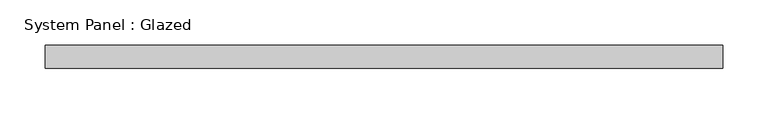
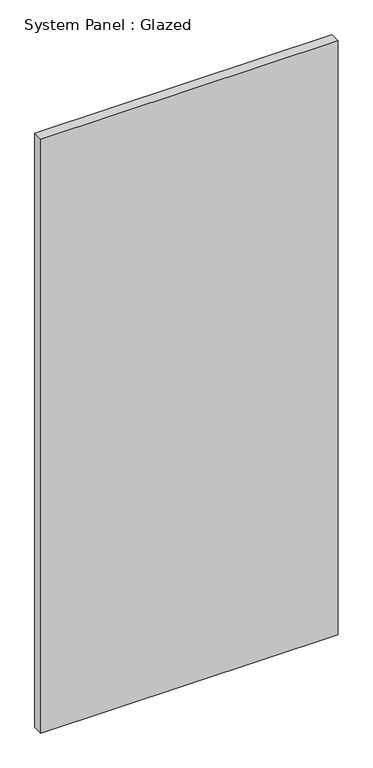
"""IFC4 building model written with IfcOpenShell, lengths in millimetres: plate geometry, System Panel : Glazed."""

from ifc_helpers import new_model, si_unit, origin, origin_with_axes, place, context, project, spatial, polyline, outline, extrude, source, transform, mapped, element, save


def system_panel_glazed_f84acb07(model_context):
    return source(origin(), model_context, "Body", "SweptSolid", [
        extrude(outline(polyline([(374.65, 19.05), (-374.65, 19.05), (-374.65, 44.45), (374.65, 44.45), (374.65, 19.05)])), origin_with_axes(), (0.0, 0.0, 1.0), 1581.8911809),
    ])


if __name__ == "__main__":
    model = new_model("IFC4")
    model_context = context("Model", 3, world=origin())
    ifc_project = project(units=[si_unit("LENGTHUNIT", "METRE", prefix="MILLI")], contexts=[model_context])
    site = spatial("IfcSite", under=ifc_project)
    building = spatial("IfcBuilding", under=site)
    placement = place(None, origin())
    system_panel_glazed_shape = system_panel_glazed_f84acb07(model_context)
    element("IfcPlate", 1, ObjectType="System Panel : Glazed", at=placement, inside=building, context=model_context, shape_type="MappedRepresentation", body=[
        mapped(system_panel_glazed_shape, transform((0.0, 0.0, 0.0), x_axis=(1.0, 0.0, 0.0), y_axis=(0.0, 1.0, 0.0), z_axis=(0.0, 0.0, 1.0))),
    ])
    save(model, "model.ifc")

# Revit data of these elements
# Type "System Panel : Glazed"
#   Construction Type Id = "GSP4R"
#   Analytic Construction = "1/8 in Pilkington single glazing"
#   Visual Light Transmittance = 0.9
#   Solar Heat Gain Coefficient = 0.86
#   Heat Transfer Coefficient (U) = 1.18115 BTU/(h·ft²·°F)
#   Define Thermal Properties by = 1
# Element 1 (IfcPlate, "System Panel : Glazed")
#   Materials on its faces: "Glass"
# Materials
#   "Glass": class "Glass", colour RGB 0 128 192, transparency 0.75, Description = "Soda Lime Glass", Cost = 0
